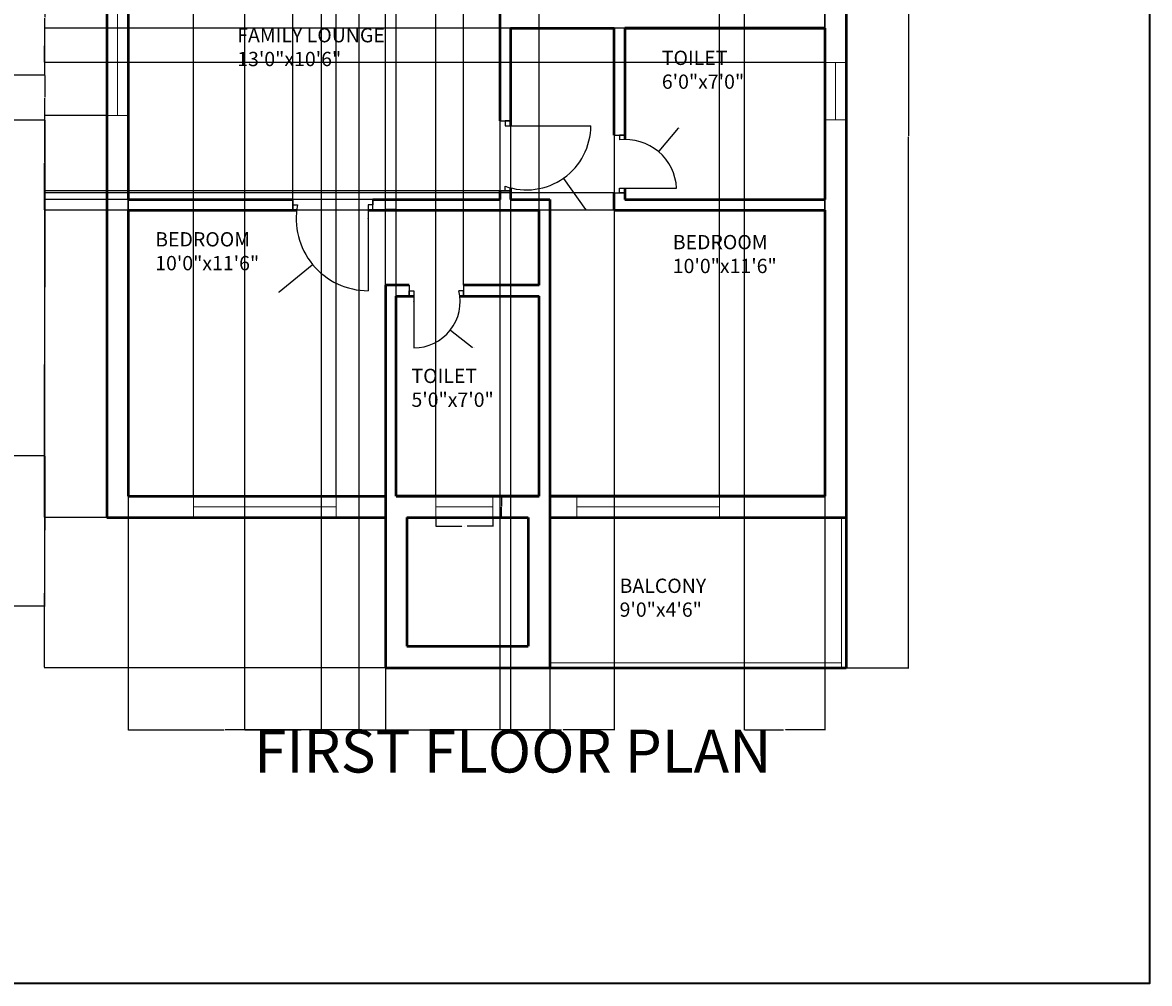
# Model space of a CAD drawing. Units: inches. Extents: x 1860 to 2753, y 1742 to 2419.
# Tile 3 of 4: x 2280 to 2753, y 1742 to 2145. Entities that reach past the tile are written whole.
import ezdxf

# ---------------------------------------------------------------- set-up
doc = ezdxf.new("R2010")
doc.units = ezdxf.units.IN
for name, color, linetype, lineweight in [('A-ANNO-DIMS', 2, 'Continuous', 18), ('A-ANNO-TEXT', 7, 'Continuous', 25), ('A-ANNO-TTLB', 7, 'Continuous', 35), ('A-AREA-IDEN', 7, 'Continuous', 18), ('A-DOOR', 3, 'Continuous', 25), ('A-FLOR-HRAL', 7, 'Continuous', 18), ('A-GLAZ', 4, 'Continuous', 18), ('A-WALL', 7, 'Continuous', 50)]:
    doc.layers.add(name, color=color, linetype=linetype, lineweight=lineweight)
doc.styles.get("Standard").update_dxf_attribs({"font": 'arial.ttf'})
doc.dimstyles.get("Standard").update_dxf_attribs({"dimtxt": 0.18, "dimasz": 0.18, "dimexe": 0.18, "dimexo": 0.0625, "dimgap": 0.09, "dimtad": 0, "dimtih": 1, "dimtoh": 1, "dimdec": 4, "dimzin": 0, "dimdsep": 46, "dimtxsty": 'Standard', "dimcen": 0.09, "dimadec": 0, "dimazin": 0, "dimtfac": 1, "dimtdec": 4, "dimtofl": 0, "dimtmove": 0, "dimatfit": 3, "dimfxl": 1, "dimtolj": 1, "dimtzin": 0, "dimarcsym": 0})

# ---------------------------------------------------------------- blocks, each defined once
blk = doc.blocks.new('WIN-24IN')
for p, q in [((0, 9), (0, 0)), ((24, 4.5), (24, 9)), ((24, 9), (24, 0)), ((0, 0), (0, 4.5)), ((0, 4.5), (24, 4.5))]:
    blk.add_line(p, q)
blk = doc.blocks.new('WIN-60IN')
for p, q in [((0, 9), (0, 0)), ((60, 4.5), (60, 9)), ((60, 9), (60, 0)), ((0, 0), (0, 4.5)), ((0, 4.5), (60, 4.5))]:
    blk.add_line(p, q)
blk = doc.blocks.new('*D5')
at = {"layer": 'A-ANNO-DIMS', "color": 0, "lineweight": -2, "transparency": 16777216}
for p, q in [((2453.69, 1937.09), (2453.69, 1933.37)), ((2477.69, 1937.09), (2477.69, 1933.37)), ((2453.87, 1933.55), (2464.58, 1933.55)), ((2477.51, 1933.55), (2466.81, 1933.55))]:
    blk.add_line(p, q, dxfattribs=at)
at = {"layer": 'A-ANNO-DIMS', "color": 0, "transparency": 16777216}
for points in [[(2453.87, 1933.58), (2453.87, 1933.52), (2453.69, 1933.55)], [(2477.51, 1933.58), (2477.51, 1933.52), (2477.69, 1933.55)]]:
    blk.add_solid(points, dxfattribs=at)
at = {"layer": 'Defpoints', "color": 0, "transparency": 16777216}
for p in [(2453.69, 1937.15), (2477.69, 1937.15), (2477.69, 1933.55)]:
    blk.add_point(p, dxfattribs=at)
at = {"layer": 'A-ANNO-DIMS', "color": 0, "transparency": 16777216, "insert": (2465.69, 1933.55), "char_height": 0.18, "attachment_point": 5}
blk.add_mtext('\\A1;WINDOW 24 TYP.', dxfattribs=at)
blk = doc.blocks.new('*D6')
at = {"layer": 'A-ANNO-DIMS', "color": 0, "lineweight": -2, "transparency": 16777216}
for p, q in [((2477.76, 1946.15), (2481.47, 1946.15)), ((2481.29, 1945.97), (2481.29, 1941.83)), ((2481.29, 1937.33), (2481.29, 1941.47)), ((2477.76, 1937.15), (2481.47, 1937.15))]:
    blk.add_line(p, q, dxfattribs=at)
at = {"layer": 'A-ANNO-DIMS', "color": 0, "transparency": 16777216}
for points in [[(2481.26, 1945.97), (2481.32, 1945.97), (2481.29, 1946.15)], [(2481.26, 1937.33), (2481.32, 1937.33), (2481.29, 1937.15)]]:
    blk.add_solid(points, dxfattribs=at)
at = {"layer": 'Defpoints', "color": 0, "transparency": 16777216}
for p in [(2477.69, 1946.15), (2481.29, 1946.15), (2477.69, 1937.15)]:
    blk.add_point(p, dxfattribs=at)
at = {"layer": 'A-ANNO-DIMS', "color": 0, "transparency": 16777216, "insert": (2481.29, 1941.65), "char_height": 0.18, "attachment_point": 5}
blk.add_mtext('\\A1;9 TYP.', dxfattribs=at)
blk = doc.blocks.new('*D17')
at = {"layer": 'A-ANNO-DIMS', "color": 0, "lineweight": -2, "transparency": 16777216}
for p, q in [((2254.53, 1963.15), (2289.75, 1963.15)), ((2289.57, 1962.97), (2289.57, 1931.83)), ((2289.57, 1900.33), (2289.57, 1931.47)), ((2263.53, 1900.15), (2289.75, 1900.15))]:
    blk.add_line(p, q, dxfattribs=at)
at = {"layer": 'A-ANNO-DIMS', "color": 0, "transparency": 16777216}
for points in [[(2289.54, 1962.97), (2289.6, 1962.97), (2289.57, 1963.15)], [(2289.54, 1900.33), (2289.6, 1900.33), (2289.57, 1900.15)]]:
    blk.add_solid(points, dxfattribs=at)
at = {"layer": 'Defpoints', "color": 0, "transparency": 16777216}
for p in [(2254.47, 1963.15), (2289.57, 1963.15), (2263.47, 1900.15)]:
    blk.add_point(p, dxfattribs=at)
at = {"layer": 'A-ANNO-DIMS', "color": 0, "transparency": 16777216, "insert": (2289.57, 1931.65), "char_height": 0.18, "attachment_point": 5}
blk.add_mtext('\\A1;63', dxfattribs=at)
blk = doc.blocks.new('*D18')
at = {"layer": 'A-ANNO-DIMS', "color": 0, "lineweight": -2, "transparency": 16777216}
for p, q in [((2254.53, 2104.15), (2289.75, 2104.15)), ((2289.57, 2103.97), (2289.57, 2033.83)), ((2289.57, 1963.33), (2289.57, 2033.47)), ((2254.53, 1963.15), (2289.75, 1963.15))]:
    blk.add_line(p, q, dxfattribs=at)
at = {"layer": 'A-ANNO-DIMS', "color": 0, "transparency": 16777216}
for points in [[(2289.54, 2103.97), (2289.6, 2103.97), (2289.57, 2104.15)], [(2289.54, 1963.33), (2289.6, 1963.33), (2289.57, 1963.15)]]:
    blk.add_solid(points, dxfattribs=at)
at = {"layer": 'Defpoints', "color": 0, "transparency": 16777216}
for p in [(2254.47, 2104.15), (2289.57, 2104.15), (2254.47, 1963.15)]:
    blk.add_point(p, dxfattribs=at)
at = {"layer": 'A-ANNO-DIMS', "color": 0, "transparency": 16777216, "insert": (2289.57, 2033.65), "char_height": 0.18, "attachment_point": 5}
blk.add_mtext('\\A1;141', dxfattribs=at)
blk = doc.blocks.new('*D19')
at = {"layer": 'A-ANNO-DIMS', "color": 0, "lineweight": -2, "transparency": 16777216}
for p, q in [((2263.53, 2122.97), (2289.75, 2122.97)), ((2289.57, 2122.79), (2289.57, 2113.74)), ((2289.57, 2104.33), (2289.57, 2113.38)), ((2254.53, 2104.15), (2289.75, 2104.15))]:
    blk.add_line(p, q, dxfattribs=at)
at = {"layer": 'A-ANNO-DIMS', "color": 0, "transparency": 16777216}
for points in [[(2289.54, 2122.79), (2289.6, 2122.79), (2289.57, 2122.97)], [(2289.54, 2104.33), (2289.6, 2104.33), (2289.57, 2104.15)]]:
    blk.add_solid(points, dxfattribs=at)
at = {"layer": 'Defpoints', "color": 0, "transparency": 16777216}
for p in [(2263.47, 2122.97), (2289.57, 2122.97), (2254.47, 2104.15)]:
    blk.add_point(p, dxfattribs=at)
at = {"layer": 'A-ANNO-DIMS', "color": 0, "transparency": 16777216, "insert": (2289.57, 2113.56), "char_height": 0.18, "attachment_point": 5}
blk.add_mtext('\\A1;18.82', dxfattribs=at)
blk = doc.blocks.new('*D20')
at = {"layer": 'A-ANNO-DIMS', "color": 0, "lineweight": -2, "transparency": 16777216}
for p, q in [((2263.53, 2170.97), (2289.75, 2170.97)), ((2289.57, 2170.79), (2289.57, 2147.15)), ((2289.57, 2123.15), (2289.57, 2146.79)), ((2263.53, 2122.97), (2289.75, 2122.97))]:
    blk.add_line(p, q, dxfattribs=at)
at = {"layer": 'A-ANNO-DIMS', "color": 0, "transparency": 16777216}
for points in [[(2289.54, 2170.79), (2289.6, 2170.79), (2289.57, 2170.97)], [(2289.54, 2123.15), (2289.6, 2123.15), (2289.57, 2122.97)]]:
    blk.add_solid(points, dxfattribs=at)
at = {"layer": 'Defpoints', "color": 0, "transparency": 16777216}
for p in [(2263.47, 2170.97), (2289.57, 2170.97), (2263.47, 2122.97)]:
    blk.add_point(p, dxfattribs=at)
at = {"layer": 'A-ANNO-DIMS', "color": 0, "transparency": 16777216, "insert": (2289.57, 2146.97), "char_height": 0.18, "attachment_point": 5}
blk.add_mtext('\\A1;48', dxfattribs=at)
blk = doc.blocks.new('*D32')
at = {"layer": 'A-ANNO-DIMS', "color": 0, "lineweight": -2, "transparency": 16777216}
for p, q in [((2626.09, 2320.15), (2652.31, 2320.15)), ((2652.13, 2319.97), (2652.13, 2097.33)), ((2652.13, 1874.33), (2652.13, 2096.97)), ((2626.09, 1874.15), (2652.31, 1874.15))]:
    blk.add_line(p, q, dxfattribs=at)
at = {"layer": 'A-ANNO-DIMS', "color": 0, "transparency": 16777216}
for points in [[(2652.1, 2319.97), (2652.16, 2319.97), (2652.13, 2320.15)], [(2652.1, 1874.33), (2652.16, 1874.33), (2652.13, 1874.15)]]:
    blk.add_solid(points, dxfattribs=at)
at = {"layer": 'Defpoints', "color": 0, "transparency": 16777216}
for p in [(2626.03, 2320.15), (2652.13, 2320.15), (2626.03, 1874.15)]:
    blk.add_point(p, dxfattribs=at)
at = {"layer": 'A-ANNO-DIMS', "color": 0, "transparency": 16777216, "insert": (2652.13, 2097.15), "char_height": 0.18, "attachment_point": 5}
blk.add_mtext('\\A1;446', dxfattribs=at)
blk = doc.blocks.new('*D33')
at = {"layer": 'A-ANNO-DIMS', "color": 0, "lineweight": -2, "transparency": 16777216}
for p, q in [((2373.33, 2311.09), (2373.33, 1847.87)), ((2421.33, 2311.09), (2421.33, 1847.87)), ((2373.51, 1848.05), (2397.11, 1848.05)), ((2421.15, 1848.05), (2397.55, 1848.05))]:
    blk.add_line(p, q, dxfattribs=at)
at = {"layer": 'A-ANNO-DIMS', "color": 0, "transparency": 16777216}
for points in [[(2373.51, 1848.08), (2373.51, 1848.02), (2373.33, 1848.05)], [(2421.15, 1848.08), (2421.15, 1848.02), (2421.33, 1848.05)]]:
    blk.add_solid(points, dxfattribs=at)
at = {"layer": 'Defpoints', "color": 0, "transparency": 16777216}
for p in [(2373.33, 2311.15), (2421.33, 2311.15), (2421.33, 1848.05)]:
    blk.add_point(p, dxfattribs=at)
at = {"layer": 'A-ANNO-DIMS', "color": 0, "transparency": 16777216, "insert": (2397.33, 1848.05), "char_height": 0.18, "attachment_point": 5}
blk.add_mtext('\\A1;48', dxfattribs=at)
blk = doc.blocks.new('*D34')
at = {"layer": 'A-ANNO-DIMS', "color": 0, "lineweight": -2, "transparency": 16777216}
for p, q in [((2421.33, 2311.09), (2421.33, 1847.87)), ((2480.53, 2311.09), (2480.53, 1847.87)), ((2421.51, 1848.05), (2450.6, 1848.05)), ((2480.35, 1848.05), (2451.25, 1848.05))]:
    blk.add_line(p, q, dxfattribs=at)
at = {"layer": 'A-ANNO-DIMS', "color": 0, "transparency": 16777216}
for points in [[(2421.51, 1848.08), (2421.51, 1848.02), (2421.33, 1848.05)], [(2480.35, 1848.08), (2480.35, 1848.02), (2480.53, 1848.05)]]:
    blk.add_solid(points, dxfattribs=at)
at = {"layer": 'Defpoints', "color": 0, "transparency": 16777216}
for p in [(2421.33, 2311.15), (2480.53, 2311.15), (2480.53, 1848.05)]:
    blk.add_point(p, dxfattribs=at)
at = {"layer": 'A-ANNO-DIMS', "color": 0, "transparency": 16777216, "insert": (2450.93, 1848.05), "char_height": 0.18, "attachment_point": 5}
blk.add_mtext('\\A1;59.2', dxfattribs=at)
blk = doc.blocks.new('*D35')
at = {"layer": 'A-ANNO-DIMS', "color": 0, "lineweight": -2, "transparency": 16777216}
for p, q in [((2583.19, 2311.09), (2583.19, 1847.87)), ((2617.03, 2311.09), (2617.03, 1847.87)), ((2583.37, 1848.05), (2599.71, 1848.05)), ((2616.85, 1848.05), (2600.5, 1848.05))]:
    blk.add_line(p, q, dxfattribs=at)
at = {"layer": 'A-ANNO-DIMS', "color": 0, "transparency": 16777216}
for points in [[(2583.37, 1848.08), (2583.37, 1848.02), (2583.19, 1848.05)], [(2616.85, 1848.08), (2616.85, 1848.02), (2617.03, 1848.05)]]:
    blk.add_solid(points, dxfattribs=at)
at = {"layer": 'Defpoints', "color": 0, "transparency": 16777216}
for p in [(2583.19, 2311.15), (2617.03, 2311.15), (2617.03, 1848.05)]:
    blk.add_point(p, dxfattribs=at)
at = {"layer": 'A-ANNO-DIMS', "color": 0, "transparency": 16777216, "insert": (2600.11, 1848.05), "char_height": 0.18, "attachment_point": 5}
blk.add_mtext('\\A1;33.84', dxfattribs=at)
blk = doc.blocks.new('*D36')
at = {"layer": 'A-ANNO-DIMS', "color": 0, "lineweight": -2, "transparency": 16777216}
for p, q in [((2324.53, 1946.21), (2324.53, 2346.43)), ((2324.71, 2346.25), (2337.76, 2346.25)), ((2351.74, 2346.25), (2338.69, 2346.25)), ((2351.92, 1946.21), (2351.92, 2346.43))]:
    blk.add_line(p, q, dxfattribs=at)
at = {"layer": 'A-ANNO-DIMS', "color": 0, "transparency": 16777216}
for points in [[(2324.71, 2346.28), (2324.71, 2346.22), (2324.53, 2346.25)], [(2351.74, 2346.28), (2351.74, 2346.22), (2351.92, 2346.25)]]:
    blk.add_solid(points, dxfattribs=at)
at = {"layer": 'Defpoints', "color": 0, "transparency": 16777216}
for p in [(2351.92, 2346.25), (2324.53, 1946.15), (2351.92, 1946.15)]:
    blk.add_point(p, dxfattribs=at)
at = {"layer": 'A-ANNO-DIMS', "color": 0, "transparency": 16777216, "insert": (2338.22, 2346.25), "char_height": 0.18, "attachment_point": 5}
blk.add_mtext('\\A1;27.396', dxfattribs=at)
blk = doc.blocks.new('*D37')
at = {"layer": 'A-ANNO-DIMS', "color": 0, "lineweight": -2, "transparency": 16777216}
for p, q in [((2411.92, 1946.21), (2411.92, 2346.43)), ((2412.1, 2346.25), (2421.76, 2346.25)), ((2432.35, 2346.25), (2422.69, 2346.25)), ((2432.53, 1946.21), (2432.53, 2346.43))]:
    blk.add_line(p, q, dxfattribs=at)
at = {"layer": 'A-ANNO-DIMS', "color": 0, "transparency": 16777216}
for points in [[(2412.1, 2346.28), (2412.1, 2346.22), (2411.92, 2346.25)], [(2432.35, 2346.28), (2432.35, 2346.22), (2432.53, 2346.25)]]:
    blk.add_solid(points, dxfattribs=at)
at = {"layer": 'Defpoints', "color": 0, "transparency": 16777216}
for p in [(2432.53, 2346.25), (2411.92, 1946.15), (2432.53, 1946.15)]:
    blk.add_point(p, dxfattribs=at)
at = {"layer": 'A-ANNO-DIMS', "color": 0, "transparency": 16777216, "insert": (2422.22, 2346.25), "char_height": 0.18, "attachment_point": 5}
blk.add_mtext('\\A1;20.604', dxfattribs=at)
blk = doc.blocks.new('*D38')
at = {"layer": 'A-ANNO-DIMS', "color": 0, "lineweight": -2, "transparency": 16777216}
for p, q in [((2432.53, 1874.09), (2432.53, 1847.87)), ((2501.53, 1874.09), (2501.53, 1847.87)), ((2432.71, 1848.05), (2466.81, 1848.05)), ((2501.35, 1848.05), (2467.24, 1848.05))]:
    blk.add_line(p, q, dxfattribs=at)
at = {"layer": 'A-ANNO-DIMS', "color": 0, "transparency": 16777216}
for points in [[(2432.71, 1848.08), (2432.71, 1848.02), (2432.53, 1848.05)], [(2501.35, 1848.08), (2501.35, 1848.02), (2501.53, 1848.05)]]:
    blk.add_solid(points, dxfattribs=at)
at = {"layer": 'Defpoints', "color": 0, "transparency": 16777216}
for p in [(2432.53, 1874.15), (2501.53, 1874.15), (2501.53, 1848.05)]:
    blk.add_point(p, dxfattribs=at)
at = {"layer": 'A-ANNO-DIMS', "color": 0, "transparency": 16777216, "insert": (2467.03, 1848.05), "char_height": 0.18, "attachment_point": 5}
blk.add_mtext('\\A1;69', dxfattribs=at)
blk = doc.blocks.new('*D39')
at = {"layer": 'A-ANNO-DIMS', "color": 0, "lineweight": -2, "transparency": 16777216}
for p, q in [((2315.46, 1937.15), (2289.25, 1937.15)), ((2289.43, 1936.97), (2289.43, 1905.83)), ((2289.43, 1874.33), (2289.43, 1905.47)), ((2432.46, 1874.15), (2289.25, 1874.15))]:
    blk.add_line(p, q, dxfattribs=at)
at = {"layer": 'A-ANNO-DIMS', "color": 0, "transparency": 16777216}
for points in [[(2289.4, 1936.97), (2289.46, 1936.97), (2289.43, 1937.15)], [(2289.4, 1874.33), (2289.46, 1874.33), (2289.43, 1874.15)]]:
    blk.add_solid(points, dxfattribs=at)
at = {"layer": 'Defpoints', "color": 0, "transparency": 16777216}
for p in [(2289.43, 1937.15), (2315.53, 1937.15), (2432.53, 1874.15)]:
    blk.add_point(p, dxfattribs=at)
at = {"layer": 'A-ANNO-DIMS', "color": 0, "transparency": 16777216, "insert": (2289.43, 1905.65), "char_height": 0.18, "attachment_point": 5}
blk.add_mtext('\\A1;63', dxfattribs=at)
blk = doc.blocks.new('*D40')
at = {"layer": 'A-ANNO-DIMS', "color": 0, "lineweight": -2, "transparency": 16777216}
for p, q in [((2324.46, 2066.15), (2289.25, 2066.15)), ((2289.43, 2065.97), (2289.43, 2001.83)), ((2289.43, 1937.33), (2289.43, 2001.47)), ((2315.46, 1937.15), (2289.25, 1937.15))]:
    blk.add_line(p, q, dxfattribs=at)
at = {"layer": 'A-ANNO-DIMS', "color": 0, "transparency": 16777216}
for points in [[(2289.4, 2065.97), (2289.46, 2065.97), (2289.43, 2066.15)], [(2289.4, 1937.33), (2289.46, 1937.33), (2289.43, 1937.15)]]:
    blk.add_solid(points, dxfattribs=at)
at = {"layer": 'Defpoints', "color": 0, "transparency": 16777216}
for p in [(2289.43, 2066.15), (2324.53, 2066.15), (2315.53, 1937.15)]:
    blk.add_point(p, dxfattribs=at)
at = {"layer": 'A-ANNO-DIMS', "color": 0, "transparency": 16777216, "insert": (2289.43, 2001.65), "char_height": 0.18, "attachment_point": 5}
blk.add_mtext('\\A1;129', dxfattribs=at)
blk = doc.blocks.new('*D41')
at = {"layer": 'A-ANNO-DIMS', "color": 0, "lineweight": -2, "transparency": 16777216}
for p, q in [((2315.46, 2105.99), (2289.25, 2105.99)), ((2289.43, 2105.81), (2289.43, 2086.25)), ((2289.43, 2066.33), (2289.43, 2085.89)), ((2324.46, 2066.15), (2289.25, 2066.15))]:
    blk.add_line(p, q, dxfattribs=at)
at = {"layer": 'A-ANNO-DIMS', "color": 0, "transparency": 16777216}
for points in [[(2289.4, 2105.81), (2289.46, 2105.81), (2289.43, 2105.99)], [(2289.4, 2066.33), (2289.46, 2066.33), (2289.43, 2066.15)]]:
    blk.add_solid(points, dxfattribs=at)
at = {"layer": 'Defpoints', "color": 0, "transparency": 16777216}
for p in [(2289.43, 2105.99), (2315.53, 2105.99), (2324.53, 2066.15)]:
    blk.add_point(p, dxfattribs=at)
at = {"layer": 'A-ANNO-DIMS', "color": 0, "transparency": 16777216, "insert": (2289.43, 2086.07), "char_height": 0.18, "attachment_point": 5}
blk.add_mtext('\\A1;39.84', dxfattribs=at)
blk = doc.blocks.new('*D43')
at = {"layer": 'A-ANNO-DIMS', "color": 0, "lineweight": -2, "transparency": 16777216}
for p, q in [((2437.03, 1946.21), (2437.03, 2346.43)), ((2437.21, 2346.25), (2444.97, 2346.25)), ((2453.51, 2346.25), (2445.74, 2346.25)), ((2453.69, 1946.21), (2453.69, 2346.43))]:
    blk.add_line(p, q, dxfattribs=at)
at = {"layer": 'A-ANNO-DIMS', "color": 0, "transparency": 16777216}
for points in [[(2437.21, 2346.28), (2437.21, 2346.22), (2437.03, 2346.25)], [(2453.51, 2346.28), (2453.51, 2346.22), (2453.69, 2346.25)]]:
    blk.add_solid(points, dxfattribs=at)
at = {"layer": 'Defpoints', "color": 0, "transparency": 16777216}
for p in [(2453.69, 2346.25), (2437.03, 1946.15), (2453.69, 1946.15)]:
    blk.add_point(p, dxfattribs=at)
at = {"layer": 'A-ANNO-DIMS', "color": 0, "transparency": 16777216, "insert": (2445.36, 2346.25), "char_height": 0.18, "attachment_point": 5}
blk.add_mtext('\\A1;16.67', dxfattribs=at)
blk = doc.blocks.new('*D44')
at = {"layer": 'A-ANNO-DIMS', "color": 0, "lineweight": -2, "transparency": 16777216}
for p, q in [((2572.85, 1946.21), (2572.85, 2346.43)), ((2573.03, 2346.25), (2594.54, 2346.25)), ((2616.85, 2346.25), (2595.34, 2346.25)), ((2617.03, 1946.21), (2617.03, 2346.43))]:
    blk.add_line(p, q, dxfattribs=at)
at = {"layer": 'A-ANNO-DIMS', "color": 0, "transparency": 16777216}
for points in [[(2573.03, 2346.28), (2573.03, 2346.22), (2572.85, 2346.25)], [(2616.85, 2346.28), (2616.85, 2346.22), (2617.03, 2346.25)]]:
    blk.add_solid(points, dxfattribs=at)
at = {"layer": 'Defpoints', "color": 0, "transparency": 16777216}
for p in [(2617.03, 2346.25), (2572.85, 1946.15), (2617.03, 1946.15)]:
    blk.add_point(p, dxfattribs=at)
at = {"layer": 'A-ANNO-DIMS', "color": 0, "transparency": 16777216, "insert": (2594.94, 2346.25), "char_height": 0.18, "attachment_point": 5}
blk.add_mtext('\\A1;44.17', dxfattribs=at)
blk = doc.blocks.new('*D45')
at = {"layer": 'A-ANNO-DIMS', "color": 0, "lineweight": -2, "transparency": 16777216}
for p, q in [((2616.96, 2142.65), (2289.25, 2142.65)), ((2289.43, 2142.47), (2289.43, 2135.56)), ((2289.43, 2128.29), (2289.43, 2135.2)), ((2616.96, 2128.11), (2289.25, 2128.11))]:
    blk.add_line(p, q, dxfattribs=at)
at = {"layer": 'A-ANNO-DIMS', "color": 0, "transparency": 16777216}
for points in [[(2289.4, 2142.47), (2289.46, 2142.47), (2289.43, 2142.65)], [(2289.4, 2128.29), (2289.46, 2128.29), (2289.43, 2128.11)]]:
    blk.add_solid(points, dxfattribs=at)
at = {"layer": 'Defpoints', "color": 0, "transparency": 16777216}
for p in [(2617.03, 2142.65), (2289.43, 2128.11), (2617.03, 2128.11)]:
    blk.add_point(p, dxfattribs=at)
at = {"layer": 'A-ANNO-DIMS', "color": 0, "transparency": 16777216, "insert": (2289.43, 2135.38), "char_height": 0.18, "attachment_point": 5}
blk.add_mtext('\\A1;14.54', dxfattribs=at)
blk = doc.blocks.new('*D46')
at = {"layer": 'A-ANNO-DIMS', "color": 0, "lineweight": -2, "transparency": 16777216}
for p, q in [((2324.53, 2066.21), (2324.53, 2346.43)), ((2324.71, 2346.25), (2358.67, 2346.25)), ((2393.43, 2346.25), (2359.46, 2346.25)), ((2393.61, 2066.21), (2393.61, 2346.43))]:
    blk.add_line(p, q, dxfattribs=at)
at = {"layer": 'A-ANNO-DIMS', "color": 0, "transparency": 16777216}
for points in [[(2324.71, 2346.28), (2324.71, 2346.22), (2324.53, 2346.25)], [(2393.43, 2346.28), (2393.43, 2346.22), (2393.61, 2346.25)]]:
    blk.add_solid(points, dxfattribs=at)
at = {"layer": 'Defpoints', "color": 0, "transparency": 16777216}
for p in [(2393.61, 2346.25), (2324.53, 2066.15), (2393.61, 2066.15)]:
    blk.add_point(p, dxfattribs=at)
at = {"layer": 'A-ANNO-DIMS', "color": 0, "transparency": 16777216, "insert": (2359.07, 2346.25), "char_height": 0.18, "attachment_point": 5}
blk.add_mtext('\\A1;69.08', dxfattribs=at)
blk = doc.blocks.new('*D47')
at = {"layer": 'A-ANNO-DIMS', "color": 0, "lineweight": -2, "transparency": 16777216}
for p, q in [((2405.53, 2191.09), (2405.53, 1847.87)), ((2324.53, 2186.59), (2324.53, 1847.87)), ((2324.71, 1848.05), (2364.82, 1848.05)), ((2405.35, 1848.05), (2365.23, 1848.05))]:
    blk.add_line(p, q, dxfattribs=at)
at = {"layer": 'A-ANNO-DIMS', "color": 0, "transparency": 16777216}
for points in [[(2324.71, 1848.08), (2324.71, 1848.02), (2324.53, 1848.05)], [(2405.35, 1848.08), (2405.35, 1848.02), (2405.53, 1848.05)]]:
    blk.add_solid(points, dxfattribs=at)
at = {"layer": 'Defpoints', "color": 0, "transparency": 16777216}
for p in [(2405.53, 2191.15), (2324.53, 2186.65), (2405.53, 1848.05)]:
    blk.add_point(p, dxfattribs=at)
at = {"layer": 'A-ANNO-DIMS', "color": 0, "transparency": 16777216, "insert": (2365.03, 1848.05), "char_height": 0.18, "attachment_point": 5}
blk.add_mtext('\\A1;81', dxfattribs=at)
blk = doc.blocks.new('*D48')
at = {"layer": 'A-ANNO-DIMS', "color": 0, "lineweight": -2, "transparency": 16777216}
for p, q in [((2465.35, 2034.71), (2465.35, 2346.43)), ((2465.53, 2346.25), (2480.8, 2346.25)), ((2496.85, 2346.25), (2481.58, 2346.25)), ((2497.03, 2034.71), (2497.03, 2346.43))]:
    blk.add_line(p, q, dxfattribs=at)
at = {"layer": 'A-ANNO-DIMS', "color": 0, "transparency": 16777216}
for points in [[(2465.53, 2346.28), (2465.53, 2346.22), (2465.35, 2346.25)], [(2496.85, 2346.28), (2496.85, 2346.22), (2497.03, 2346.25)]]:
    blk.add_solid(points, dxfattribs=at)
at = {"layer": 'Defpoints', "color": 0, "transparency": 16777216}
for p in [(2497.03, 2346.25), (2465.35, 2034.65), (2497.03, 2034.65)]:
    blk.add_point(p, dxfattribs=at)
at = {"layer": 'A-ANNO-DIMS', "color": 0, "transparency": 16777216, "insert": (2481.19, 2346.25), "char_height": 0.18, "attachment_point": 5}
blk.add_mtext('\\A1;31.67', dxfattribs=at)
blk = doc.blocks.new('*D49')
at = {"layer": 'A-ANNO-DIMS', "color": 0, "lineweight": -2, "transparency": 16777216}
for p, q in [((2485.03, 2142.59), (2485.03, 1847.87)), ((2528.53, 2142.59), (2528.53, 1847.87)), ((2485.21, 1848.05), (2506.45, 1848.05)), ((2528.35, 1848.05), (2507.1, 1848.05))]:
    blk.add_line(p, q, dxfattribs=at)
at = {"layer": 'A-ANNO-DIMS', "color": 0, "transparency": 16777216}
for points in [[(2485.21, 1848.08), (2485.21, 1848.02), (2485.03, 1848.05)], [(2528.35, 1848.08), (2528.35, 1848.02), (2528.53, 1848.05)]]:
    blk.add_solid(points, dxfattribs=at)
at = {"layer": 'Defpoints', "color": 0, "transparency": 16777216}
for p in [(2485.03, 2142.65), (2528.53, 2142.65), (2528.53, 1848.05)]:
    blk.add_point(p, dxfattribs=at)
at = {"layer": 'A-ANNO-DIMS', "color": 0, "transparency": 16777216, "insert": (2506.78, 1848.05), "char_height": 0.18, "attachment_point": 5}
blk.add_mtext('\\A1;43.5', dxfattribs=at)
blk = doc.blocks.new('*D51')
at = {"layer": 'A-ANNO-DIMS', "color": 0, "lineweight": -2, "transparency": 16777216}
for p, q in [((2480.46, 2074.28), (2289.25, 2074.28)), ((2289.43, 2074.1), (2289.43, 2072.65)), ((2480.46, 2070.65), (2289.25, 2070.65)), ((2289.43, 2070.83), (2289.43, 2072.28))]:
    blk.add_line(p, q, dxfattribs=at)
at = {"layer": 'A-ANNO-DIMS', "color": 0, "transparency": 16777216}
for points in [[(2289.4, 2074.1), (2289.46, 2074.1), (2289.43, 2074.28)], [(2289.4, 2070.83), (2289.46, 2070.83), (2289.43, 2070.65)]]:
    blk.add_solid(points, dxfattribs=at)
at = {"layer": 'Defpoints', "color": 0, "transparency": 16777216}
for p in [(2289.43, 2074.28), (2480.53, 2074.28), (2480.53, 2070.65)]:
    blk.add_point(p, dxfattribs=at)
at = {"layer": 'A-ANNO-DIMS', "color": 0, "transparency": 16777216, "insert": (2289.43, 2072.46), "char_height": 0.18, "attachment_point": 5}
blk.add_mtext('\\A1;3.634', dxfattribs=at)
blk = doc.blocks.new('*D52')
at = {"layer": 'A-ANNO-DIMS', "color": 0, "lineweight": -2, "transparency": 16777216}
for p, q in [((2528.46, 2073.42), (2289.25, 2073.42)), ((2289.43, 2073.24), (2289.43, 2069.96)), ((2289.43, 2066.33), (2289.43, 2069.6)), ((2528.46, 2066.15), (2289.25, 2066.15))]:
    blk.add_line(p, q, dxfattribs=at)
at = {"layer": 'A-ANNO-DIMS', "color": 0, "transparency": 16777216}
for points in [[(2289.4, 2073.24), (2289.46, 2073.24), (2289.43, 2073.42)], [(2289.4, 2066.33), (2289.46, 2066.33), (2289.43, 2066.15)]]:
    blk.add_solid(points, dxfattribs=at)
at = {"layer": 'Defpoints', "color": 0, "transparency": 16777216}
for p in [(2289.43, 2073.42), (2528.53, 2073.42), (2528.53, 2066.15)]:
    blk.add_point(p, dxfattribs=at)
at = {"layer": 'A-ANNO-DIMS', "color": 0, "transparency": 16777216, "insert": (2289.43, 2069.78), "char_height": 0.18, "attachment_point": 5}
blk.add_mtext('\\A1;7.268', dxfattribs=at)
blk = doc.blocks.new('*D56')
at = {"layer": 'A-ANNO-DIMS', "color": 0, "lineweight": -2, "transparency": 16777216}
for p, q in [((2425.22, 2062.65), (2425.4, 2062.65)), ((2425.31, 2062.56), (2425.31, 2062.74)), ((2387.97, 2031.85), (2401.83, 2043.28)), ((2387.79, 2031.85), (2387.97, 2031.85))]:
    blk.add_line(p, q, dxfattribs=at)
at = {"layer": 'A-ANNO-DIMS', "color": 0, "transparency": 16777216}
blk.add_solid([(2401.81, 2043.31), (2401.85, 2043.26), (2401.97, 2043.4)], dxfattribs=at)
at = {"layer": 'Defpoints', "color": 0, "transparency": 16777216}
for p in [(2425.31, 2062.65), (2401.97, 2043.4)]:
    blk.add_point(p, dxfattribs=at)
at = {"layer": 'A-ANNO-DIMS', "color": 0, "transparency": 16777216, "insert": (2387.31, 2031.85), "char_height": 0.18, "attachment_point": 5}
blk.add_mtext('\\A1;R30.25', dxfattribs=at)
blk = doc.blocks.new('*D58')
at = {"layer": 'A-ANNO-DIMS', "color": 0, "lineweight": -2, "transparency": 16777216}
for p, q in [((2491.74, 2101.66), (2491.92, 2101.66)), ((2491.83, 2101.57), (2491.83, 2101.75)), ((2516.67, 2066.43), (2507.46, 2079.49)), ((2516.85, 2066.43), (2516.67, 2066.43))]:
    blk.add_line(p, q, dxfattribs=at)
at = {"layer": 'A-ANNO-DIMS', "color": 0, "transparency": 16777216}
blk.add_solid([(2507.48, 2079.51), (2507.43, 2079.48), (2507.36, 2079.64)], dxfattribs=at)
at = {"layer": 'Defpoints', "color": 0, "transparency": 16777216}
for p in [(2491.83, 2101.66), (2507.36, 2079.64)]:
    blk.add_point(p, dxfattribs=at)
at = {"layer": 'A-ANNO-DIMS', "color": 0, "transparency": 16777216, "insert": (2517.33, 2066.43), "char_height": 0.18, "attachment_point": 5}
blk.add_mtext('\\A1;R26.95', dxfattribs=at)
blk = doc.blocks.new('*D59')
at = {"layer": 'A-ANNO-DIMS', "color": 0, "lineweight": -2, "transparency": 16777216}
for p, q in [((2555.47, 2100.59), (2547.31, 2090.91)), ((2555.65, 2100.59), (2555.47, 2100.59)), ((2533.32, 2074.42), (2533.5, 2074.42)), ((2533.41, 2074.33), (2533.41, 2074.51))]:
    blk.add_line(p, q, dxfattribs=at)
at = {"layer": 'A-ANNO-DIMS', "color": 0, "transparency": 16777216}
blk.add_solid([(2547.29, 2090.93), (2547.33, 2090.89), (2547.2, 2090.78)], dxfattribs=at)
at = {"layer": 'Defpoints', "color": 0, "transparency": 16777216}
for p in [(2547.2, 2090.78), (2533.41, 2074.42)]:
    blk.add_point(p, dxfattribs=at)
at = {"layer": 'A-ANNO-DIMS', "color": 0, "transparency": 16777216, "insert": (2556.13, 2100.59), "char_height": 0.18, "attachment_point": 5}
blk.add_mtext('\\A1;R21.39', dxfattribs=at)
blk = doc.blocks.new('*D60')
at = {"layer": 'A-ANNO-DIMS', "color": 0, "lineweight": -2, "transparency": 16777216}
for p, q in [((2444.4, 2027.81), (2444.58, 2027.81)), ((2444.49, 2027.72), (2444.49, 2027.9)), ((2468.91, 2008.61), (2459.89, 2015.7)), ((2469.09, 2008.61), (2468.91, 2008.61))]:
    blk.add_line(p, q, dxfattribs=at)
at = {"layer": 'A-ANNO-DIMS', "color": 0, "transparency": 16777216}
blk.add_solid([(2459.91, 2015.73), (2459.87, 2015.68), (2459.75, 2015.81)], dxfattribs=at)
at = {"layer": 'Defpoints', "color": 0, "transparency": 16777216}
for p in [(2444.49, 2027.81), (2459.75, 2015.81)]:
    blk.add_point(p, dxfattribs=at)
at = {"layer": 'A-ANNO-DIMS', "color": 0, "transparency": 16777216, "insert": (2469.64, 2008.61), "char_height": 0.18, "attachment_point": 5}
blk.add_mtext('\\A1;R19.417', dxfattribs=at)

msp = doc.modelspace()

# ---------------------------------------------------------------- linework, layer by layer
at = {"layer": 'A-ANNO-TTLB'}
msp.add_lwpolyline([(1859.5561, 2419.29), (2753.3204, 2419.29), (2753.3204, 1741.6035), (1859.5561, 1741.6035)], close=True, dxfattribs=at)
at = {"layer": 'A-DOOR'}
for p, q in [((2480.525, 2103.664), (2485.025, 2103.664)), ((2485.025, 2103.664), (2482.775, 2103.664)), ((2482.775, 2103.664), (2482.775, 2101.664)), ((2482.775, 2101.664), (2518.775, 2101.664)), ((2528.525, 2097.6491), (2533.025, 2097.6491)), ((2533.025, 2097.6491), (2530.775, 2097.6491)), ((2530.775, 2097.6491), (2530.775, 2095.6491)), ((2480.525, 2074.2818), (2485.025, 2074.2818)), ((2485.025, 2074.2818), (2480.525, 2074.2818)), ((2480.525, 2074.2818), (2482.775, 2074.2818)), ((2482.775, 2074.2818), (2482.775, 2076.2818)), ((2528.525, 2073.4157), (2533.025, 2073.4157)), ((2530.775, 2073.4157), (2530.775, 2075.4157)), ((2530.775, 2075.4157), (2554.775, 2075.4157)), ((2533.025, 2073.4157), (2530.775, 2073.4157)), ((2393.6072, 2070.6476), (2393.6072, 2066.1476)), ((2393.6072, 2066.1476), (2393.6072, 2068.3976)), ((2393.6072, 2068.3976), (2395.6072, 2068.3976)), ((2427.3075, 2068.3976), (2425.3075, 2068.3976)), ((2425.3075, 2068.3976), (2425.3075, 2032.3976)), ((2427.3075, 2066.1476), (2427.3075, 2070.6476)), ((2427.3075, 2070.6476), (2427.3075, 2068.3976)), ((2442.4863, 2034.6476), (2442.4863, 2030.1476)), ((2465.355, 2034.6476), (2465.355, 2030.1476)), ((2442.4863, 2030.1476), (2442.4863, 2032.3976)), ((2442.4863, 2032.3976), (2444.4863, 2032.3976)), ((2442.4863, 2030.1476), (2442.4863, 2030.1476)), ((2444.4863, 2032.3976), (2444.4863, 2008.3976)), ((2465.355, 2032.3976), (2463.355, 2032.3976)), ((2465.355, 2030.1476), (2465.355, 2032.3976))]:
    msp.add_line(p, q, dxfattribs=at)
for centre, radius, start, end in [((2491.827, 2101.664), 26.948, 250.372234, 0), ((2533.4086, 2074.4224), 21.3894, 2.661671, 97.07263), ((2425.3075, 2062.6491), 30.2515, 169.045821, 270), ((2444.4863, 2027.8148), 19.4172, 270, 13.651636)]:
    msp.add_arc(centre, radius, start, end, dxfattribs=at)
at = {"layer": 'A-FLOR-HRAL'}
for p, q in [((2626.025, 1937.1476), (2624.025, 1937.1476)), ((2624.025, 1937.1476), (2624.025, 1874.1476)), ((2624.025, 1876.1476), (2501.525, 1876.1476)), ((2624.025, 1874.1476), (2624.025, 1876.1476))]:
    msp.add_line(p, q, dxfattribs=at)
at = {"layer": 'A-GLAZ'}
for p, q in [((2411.9209, 1937.1476), (2411.9209, 1937.1476)), ((2572.854, 1937.1476), (2572.854, 1937.1476))]:
    msp.add_line(p, q, dxfattribs=at)
at = {"layer": 'A-WALL'}
for p, q in [((2315.525, 2320.1476), (2315.525, 1937.1476)), ((2626.025, 2320.1476), (2626.025, 1874.1476)), ((2324.525, 2186.6476), (2324.525, 2070.6476)), ((2480.525, 2151.1172), (2480.525, 2103.664)), ((2485.025, 2142.6476), (2528.525, 2142.6476)), ((2485.025, 2142.6476), (2485.025, 2101.664)), ((2528.525, 2097.6491), (2528.525, 2142.6476)), ((2617.025, 2142.6476), (2533.025, 2142.6476)), ((2533.025, 2142.6476), (2533.025, 2095.8084)), ((2533.025, 2142.6476), (2617.025, 2142.6476)), ((2617.025, 2142.6476), (2617.025, 2070.6476)), ((2480.525, 2074.2818), (2480.525, 2070.6476)), ((2485.025, 2075.5886), (2485.025, 2070.6476)), ((2528.525, 2066.1476), (2528.525, 2073.4157)), ((2533.025, 2075.4157), (2533.025, 2070.6476)), ((2324.525, 2070.6476), (2393.6072, 2070.6476)), ((2427.3075, 2070.6476), (2480.525, 2070.6476)), ((2485.025, 2070.6476), (2501.525, 2070.6476)), ((2501.525, 2070.6476), (2501.525, 1874.1476)), ((2533.025, 2070.6476), (2533.025, 2070.6476)), ((2533.025, 2070.6476), (2617.025, 2070.6476)), ((2324.525, 2066.1476), (2395.259, 2066.1476)), ((2324.525, 2066.1476), (2324.525, 1946.1476)), ((2425.3075, 2066.1476), (2497.025, 2066.1476)), ((2437.025, 2066.1476), (2432.525, 2066.1476)), ((2485.025, 2066.1476), (2497.025, 2066.1476)), ((2497.025, 2034.6476), (2497.025, 2066.1476)), ((2528.525, 2066.1476), (2617.025, 2066.1476)), ((2528.525, 2066.1476), (2617.025, 2066.1476)), ((2617.025, 2066.1476), (2617.025, 1946.1476)), ((2432.525, 2034.6476), (2432.525, 1874.1476)), ((2442.4863, 2034.6476), (2432.525, 2034.6476)), ((2497.025, 2034.6476), (2465.355, 2034.6476)), ((2437.025, 1946.1476), (2437.025, 2030.1476)), ((2437.025, 1946.1476), (2437.025, 2030.1476)), ((2437.025, 2030.1476), (2444.4863, 2030.1476)), ((2463.7629, 2030.1476), (2497.025, 2030.1476)), ((2497.025, 1946.1476), (2497.025, 2030.1476)), ((2324.525, 1946.1476), (2432.525, 1946.1476)), ((2497.025, 1946.1476), (2437.025, 1946.1476)), ((2437.025, 1946.1476), (2497.025, 1946.1476)), ((2617.025, 1946.1476), (2501.525, 1946.1476)), ((2501.525, 1946.1476), (2617.025, 1946.1476)), ((2315.525, 1937.1476), (2432.525, 1937.1476)), ((2441.525, 1937.1476), (2441.525, 1883.1476)), ((2441.525, 1937.1476), (2492.525, 1937.1476)), ((2492.525, 1937.1476), (2492.525, 1883.1476)), ((2501.525, 1937.1476), (2626.025, 1937.1476)), ((2441.525, 1883.1476), (2492.525, 1883.1476)), ((2432.525, 1874.1476), (2626.025, 1874.1476))]:
    msp.add_line(p, q, dxfattribs=at)

# ---------------------------------------------------------------- block references
at = {"layer": 'A-GLAZ', "rotation": 270.0000000000017}
msp.add_blockref('WIN-60IN', (2315.525, 2165.9892), dxfattribs=at)
at = {"layer": 'A-GLAZ', "extrusion": (0, 0, -1), "zscale": -1, "rotation": 269.9999999999974}
msp.add_blockref('WIN-24IN', (-2626.025, 2128.109), dxfattribs=at)
at = {"layer": 'A-GLAZ', "extrusion": (0, 0, -1), "zscale": -1}
msp.add_blockref('WIN-60IN', (-2411.9209, 1937.1476), dxfattribs=at)
at = {"layer": 'A-GLAZ'}
for name, p in [('WIN-24IN', (2453.6944, 1937.1476)), ('WIN-60IN', (2512.854, 1937.1476))]:
    msp.add_blockref(name, p, dxfattribs=at)

# ---------------------------------------------------------------- texts
at = {"layer": 'A-ANNO-TEXT', "insert": (2377.4301, 1848.1393), "char_height": 18, "attachment_point": 1}
msp.add_mtext_dynamic_manual_height_columns('FIRST FLOOR PLAN ', width=301.732135, gutter_width=12.5, heights=[0], dxfattribs=at)
at = {"layer": 'A-AREA-IDEN', "char_height": 6, "attachment_point": 1}
for s, width, insert in [('FAMILY LOUNGE\\P13\'0"x10\'6"', 140.478597, (2370.3272, 2142.6476)), ('TOILET\\P6\'0"x7\'0"', 129.374954, (2548.5975, 2133.1347)), ('BEDROOM\\P10\'0"x11\'6"', 135.759499, (2335.8906, 2056.9628)), ('BEDROOM\\P10\'0"x11\'6"', 148.175104, (2553.1866, 2055.7758)), ('TOILET\\P5\'0"x7\'0"', 70.289955, (2443.4716, 1999.6339)), ('BALCONY\\P9\'0"x4\'6"', 142.164719, (2530.8522, 1911.5284))]:
    msp.add_mtext_dynamic_manual_height_columns(s, width=width, gutter_width=12.5, heights=[0], dxfattribs=dict(at, insert=insert))

# ---------------------------------------------------------------- dimensions: what is measured, and where the dimension line sits
at = {"layer": 'A-ANNO-DIMS'}
for base, p1, p2, override, picture, middle in [((2351.9209, 2346.2476), (2324.525, 1946.1476), (2351.9209, 1946.1476), {"dimdec": 3, "dimlfac": 1, "dimrnd": 0, "dimzin": 0, "dimdsep": 46, "dimlunit": 2}, '*D36', (2338.223, 2346.2476)), ((2393.6072, 2346.2476), (2324.525, 2066.1476), (2393.6072, 2066.1476), {"dimdec": 2, "dimlfac": 1, "dimrnd": 0, "dimzin": 0, "dimdsep": 46, "dimlunit": 2}, '*D46', (2359.0661, 2346.2476)), ((2432.525, 2346.2476), (2411.9209, 1946.1476), (2432.525, 1946.1476), {"dimdec": 3, "dimlfac": 1, "dimrnd": 0, "dimzin": 0, "dimdsep": 46, "dimlunit": 2}, '*D37', (2422.223, 2346.2476)), ((2453.6944, 2346.2476), (2437.025, 1946.1476), (2453.6944, 1946.1476), {"dimdec": 2, "dimlfac": 1, "dimrnd": 0, "dimzin": 0, "dimdsep": 46, "dimlunit": 2}, '*D43', (2445.3597, 2346.2476)), ((2497.025, 2346.2476), (2465.355, 2034.6476), (2497.025, 2034.6476), {"dimdec": 2, "dimlfac": 1, "dimrnd": 0, "dimzin": 0, "dimdsep": 46, "dimlunit": 2}, '*D48', (2481.19, 2346.2476)), ((2617.025, 2346.2476), (2572.854, 1946.1476), (2617.025, 1946.1476), {"dimdec": 2, "dimlfac": 1, "dimrnd": 0, "dimzin": 0, "dimdsep": 46, "dimlunit": 2}, '*D44', (2594.9395, 2346.2476)), ((2421.3292, 1848.0476), (2373.3292, 2311.1476), (2421.3292, 2311.1476), {"dimdec": 0, "dimlfac": 1, "dimrnd": 0, "dimzin": 0, "dimdsep": 46, "dimlunit": 2}, '*D33', (2397.3292, 1848.0476)), ((2480.525, 1848.0476), (2421.3292, 2311.1476), (2480.525, 2311.1476), {"dimdec": 1, "dimlfac": 1, "dimrnd": 0, "dimzin": 0, "dimdsep": 46, "dimlunit": 2}, '*D34', (2450.9271, 1848.0476)), ((2617.025, 1848.0476), (2583.1855, 2311.1476), (2617.025, 2311.1476), {"dimdec": 2, "dimlfac": 1, "dimrnd": 0, "dimzin": 0, "dimdsep": 46, "dimlunit": 2}, '*D35', (2600.1053, 1848.0476)), ((2405.525, 1848.0476), (2324.525, 2186.6476), (2405.525, 2191.1476), {"dimdec": 0, "dimlfac": 1, "dimrnd": 0, "dimzin": 0, "dimdsep": 46, "dimlunit": 2}, '*D47', (2365.025, 1848.0476)), ((2528.525, 1848.0476), (2485.025, 2142.6476), (2528.525, 2142.6476), {"dimdec": 1, "dimlfac": 1, "dimrnd": 0, "dimzin": 0, "dimdsep": 46, "dimlunit": 2}, '*D49', (2506.775, 1848.0476)), ((2501.525, 1848.0476), (2432.525, 1874.1476), (2501.525, 1874.1476), {"dimdec": 0, "dimlfac": 1, "dimrnd": 0, "dimzin": 0, "dimdsep": 46, "dimlunit": 2}, '*D38', (2467.025, 1848.0476))]:
    dim = msp.add_linear_dim(base=base, p1=p1, p2=p2, dimstyle='Standard', override=override, dxfattribs=at)
    dim.commit()
    dim.dimension.update_dxf_attribs({"geometry": picture, "text_midpoint": middle})
for base, p1, p2, override, picture, middle in [((2652.125, 2320.1476), (2626.025, 1874.1476), (2626.025, 2320.1476), {"dimdec": 0, "dimlfac": 1, "dimrnd": 0, "dimzin": 0, "dimdsep": 46, "dimlunit": 2}, '*D32', (2652.125, 2097.1476)), ((2289.5703, 2170.9674), (2263.4703, 2122.9674), (2263.4703, 2170.9674), {"dimdec": 0, "dimlfac": 1, "dimrnd": 0, "dimzin": 0, "dimdsep": 46, "dimlunit": 2}, '*D20', (2289.5703, 2146.9674)), ((2289.425, 2128.109), (2617.025, 2142.6476), (2617.025, 2128.109), {"dimdec": 2, "dimlfac": 1, "dimrnd": 0, "dimzin": 0, "dimdsep": 46, "dimlunit": 2}, '*D45', (2289.425, 2135.3783)), ((2289.5703, 2122.9674), (2254.4703, 2104.1476), (2263.4703, 2122.9674), {"dimdec": 2, "dimlfac": 1, "dimrnd": 0, "dimzin": 0, "dimdsep": 46, "dimlunit": 2}, '*D19', (2289.5703, 2113.5575)), ((2289.425, 2105.9892), (2324.525, 2066.1476), (2315.525, 2105.9892), {"dimdec": 2, "dimlfac": 1, "dimrnd": 0, "dimzin": 0, "dimdsep": 46, "dimlunit": 2}, '*D41', (2289.425, 2086.0684)), ((2289.5703, 2104.1476), (2254.4703, 1963.1476), (2254.4703, 2104.1476), {"dimdec": 0, "dimlfac": 1, "dimrnd": 0, "dimzin": 0, "dimdsep": 46, "dimlunit": 2}, '*D18', (2289.5703, 2033.6476)), ((2289.425, 2074.2818), (2480.525, 2070.6476), (2480.525, 2074.2818), {"dimdec": 3, "dimlfac": 1, "dimrnd": 0, "dimzin": 0, "dimdsep": 46, "dimlunit": 2}, '*D51', (2289.425, 2072.4647)), ((2289.425, 2073.4157), (2528.525, 2066.1476), (2528.525, 2073.4157), {"dimdec": 3, "dimlfac": 1, "dimrnd": 0, "dimzin": 0, "dimdsep": 46, "dimlunit": 2}, '*D52', (2289.425, 2069.7817)), ((2289.425, 2066.1476), (2315.525, 1937.1476), (2324.525, 2066.1476), {"dimdec": 0, "dimlfac": 1, "dimrnd": 0, "dimzin": 0, "dimdsep": 46, "dimlunit": 2}, '*D40', (2289.425, 2001.6476)), ((2289.5703, 1963.1476), (2263.4703, 1900.1476), (2254.4703, 1963.1476), {"dimdec": 0, "dimlfac": 1, "dimrnd": 0, "dimzin": 0, "dimdsep": 46, "dimlunit": 2}, '*D17', (2289.5703, 1931.6476)), ((2289.425, 1937.1476), (2432.525, 1874.1476), (2315.525, 1937.1476), {"dimdec": 0, "dimlfac": 1, "dimrnd": 0, "dimzin": 0, "dimdsep": 46, "dimlunit": 2}, '*D39', (2289.425, 1905.6476))]:
    dim = msp.add_linear_dim(base=base, p1=p1, p2=p2, angle=90, dimstyle='Standard', override=override, dxfattribs=at)
    dim.commit()
    dim.dimension.update_dxf_attribs({"geometry": picture, "text_midpoint": middle})
for center, mpoint, override, picture, middle in [((2491.827, 2101.664), (2507.3552, 2079.6397), {"dimdec": 2, "dimlfac": 1, "dimrnd": 0, "dimzin": 0, "dimdsep": 46, "dimlunit": 2}, '*D58', (2517.3326, 2066.4251)), ((2533.4086, 2074.4224), (2547.1951, 2090.7761), {"dimdec": 2, "dimlfac": 1, "dimrnd": 0, "dimzin": 0, "dimdsep": 46, "dimlunit": 2}, '*D59', (2556.127, 2100.5883)), ((2425.3075, 2062.6491), (2401.9725, 2043.3974), {"dimdec": 2, "dimlfac": 1, "dimrnd": 0, "dimzin": 0, "dimdsep": 46, "dimlunit": 2}, '*D56', (2387.3109, 2031.8464)), ((2444.4863, 2027.8148), (2459.751, 2015.814), {"dimdec": 3, "dimlfac": 1, "dimrnd": 0, "dimzin": 0, "dimdsep": 46, "dimlunit": 2}, '*D60', (2469.6395, 2008.6136))]:
    dim = msp.add_radius_dim(center=center, mpoint=mpoint, dimstyle='Standard', override=override, dxfattribs=at)
    dim.commit()
    dim.dimension.update_dxf_attribs({"geometry": picture, "text_midpoint": middle, "dimtype": 164})
dim = msp.add_linear_dim(base=(2481.2944, 1946.1476), p1=(2477.6944, 1937.1476), p2=(2477.6944, 1946.1476), angle=90, text='<> TYP.', dimstyle='Standard', override={"dimdec": 0, "dimlfac": 1, "dimrnd": 0, "dimzin": 0, "dimdsep": 46, "dimlunit": 2}, dxfattribs=at)
dim.commit()
dim.dimension.update_dxf_attribs({"geometry": '*D6', "text_midpoint": (2481.2944, 1941.6476)})
dim = msp.add_linear_dim(base=(2477.6944, 1933.5476), p1=(2453.6944, 1937.1476), p2=(2477.6944, 1937.1476), text='WINDOW <> TYP.', dimstyle='Standard', override={"dimdec": 0, "dimlfac": 1, "dimrnd": 0, "dimzin": 0, "dimdsep": 46, "dimlunit": 2}, dxfattribs=at)
dim.commit()
dim.dimension.update_dxf_attribs({"geometry": '*D5', "text_midpoint": (2465.6944, 1933.5476)})

doc.saveas('drawing.dxf')
